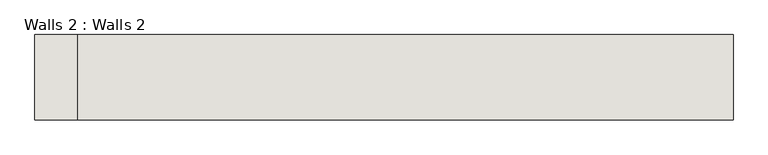
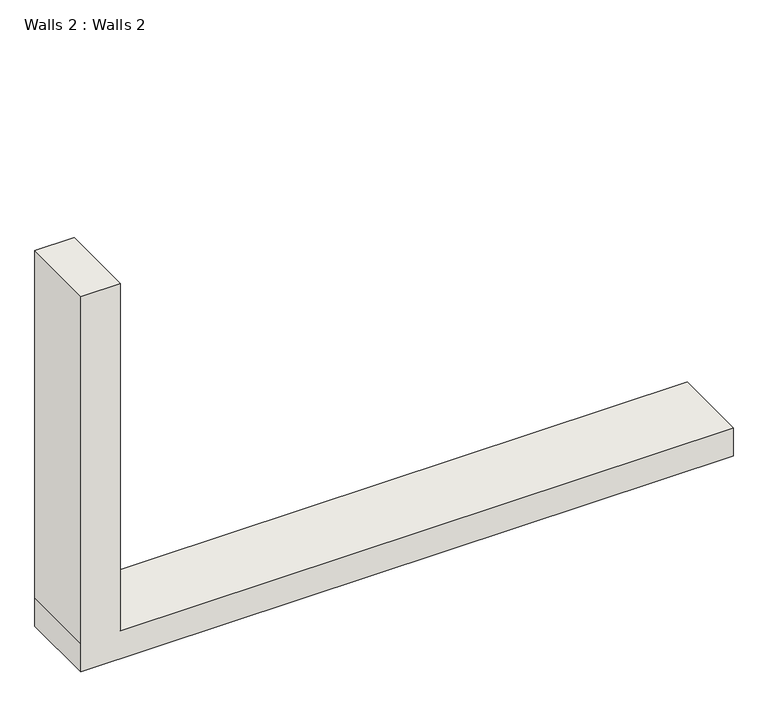
"""IFC4 building model written with IfcOpenShell, lengths in millimetres: wall geometry, Walls 2 : Walls 2."""

from ifc_helpers import new_model, si_unit, frame, origin, place, context, project, spatial, polyline, outline, extrude, source, transform, mapped, element, save


def walls_2_walls_2_db01f069(model_context):
    return source(origin(), model_context, "Body", "SweptSolid", [
        extrude(outline(polyline([(2648.0, -12313.0996792), (2648.0, -12513.0996792), (779.8738057, -12513.0996792), (627.4738057, -12513.0996792), (627.4738057, -9197.0226654), (779.8738057, -9197.0226654), (779.8738057, -12313.0996792), (2648.0, -12313.0996792)])), frame((0.0, -7794.8501996, 0.0), z_axis=(0.0, 1.0, 0.0), x_axis=(0.0, 0.0, 1.0)), (0.0, 0.0, 1.0), 404.8),
    ])


if __name__ == "__main__":
    model = new_model("IFC4")
    model_context = context("Model", 3, world=origin())
    ifc_project = project(units=[si_unit("LENGTHUNIT", "METRE", prefix="MILLI")], contexts=[model_context])
    site = spatial("IfcSite", under=ifc_project)
    building = spatial("IfcBuilding", under=site)
    placement = place(None, origin())
    walls_2_walls_2_shape = walls_2_walls_2_db01f069(model_context)
    element("IfcWall", 1, ObjectType="Walls 2 : Walls 2", at=placement, inside=building, context=model_context, shape_type="MappedRepresentation", body=[
        mapped(walls_2_walls_2_shape, transform((0.0, 0.0, 0.0), x_axis=(1.0, 0.0, 0.0), y_axis=(0.0, 1.0, 0.0), z_axis=(0.0, 0.0, 1.0))),
    ])
    save(model, "model.ifc")

# Revit data of these elements
# Element 1 (IfcWall, "Walls 2 : Walls 2")
#   Materials on its faces: "Default Wall"
# Materials
#   "Default Wall": colour RGB 80 80 80, transparency 0
